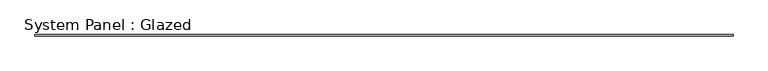
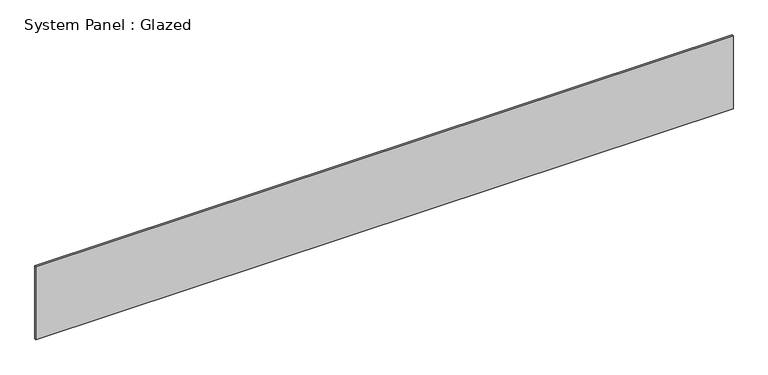
"""IFC4 building model written with IfcOpenShell, lengths in millimetres: plate geometry, System Panel : Glazed."""

from ifc_helpers import new_model, si_unit, origin, origin_with_axes, place, context, project, spatial, polyline, outline, extrude, source, transform, mapped, element, save


def system_panel_glazed_e6d06af6(model_context):
    return source(origin(), model_context, "Body", "SweptSolid", [
        extrude(outline(polyline([(6877.4735748, 19.05), (-6877.4735748, 19.05), (-6877.4735748, 44.45), (6877.4735748, 44.45), (6877.4735748, 19.05)])), origin_with_axes(), (0.0, 0.0, 1.0), 1524.0),
    ])


if __name__ == "__main__":
    model = new_model("IFC4")
    model_context = context("Model", 3, world=origin())
    ifc_project = project(units=[si_unit("LENGTHUNIT", "METRE", prefix="MILLI")], contexts=[model_context])
    site = spatial("IfcSite", under=ifc_project)
    building = spatial("IfcBuilding", under=site)
    placement = place(None, origin())
    system_panel_glazed_shape = system_panel_glazed_e6d06af6(model_context)
    element("IfcPlate", 1, ObjectType="System Panel : Glazed", at=placement, inside=building, context=model_context, shape_type="MappedRepresentation", body=[
        mapped(system_panel_glazed_shape, transform((0.0, 0.0, 0.0), x_axis=(1.0, 0.0, 0.0), y_axis=(0.0, 1.0, 0.0), z_axis=(0.0, 0.0, 1.0))),
    ])
    save(model, "model.ifc")

# Revit data of these elements
# Type "System Panel : Glazed"
#   Construction Type Id = "GSP4R"
#   Analytic Construction = "1/8 in Pilkington single glazing"
#   Visual Light Transmittance = 0.9
#   Solar Heat Gain Coefficient = 0.86
#   Heat Transfer Coefficient (U) = 1.18115 BTU/(h·ft²·°F)
# Element 1 (IfcPlate, "System Panel : Glazed")
#   Materials on its faces: "Glass"
# Materials
#   "Glass": class "Glass", colour RGB 0 128 192, transparency 0.75, Description = "Soda Lime Glass", Cost = 0
